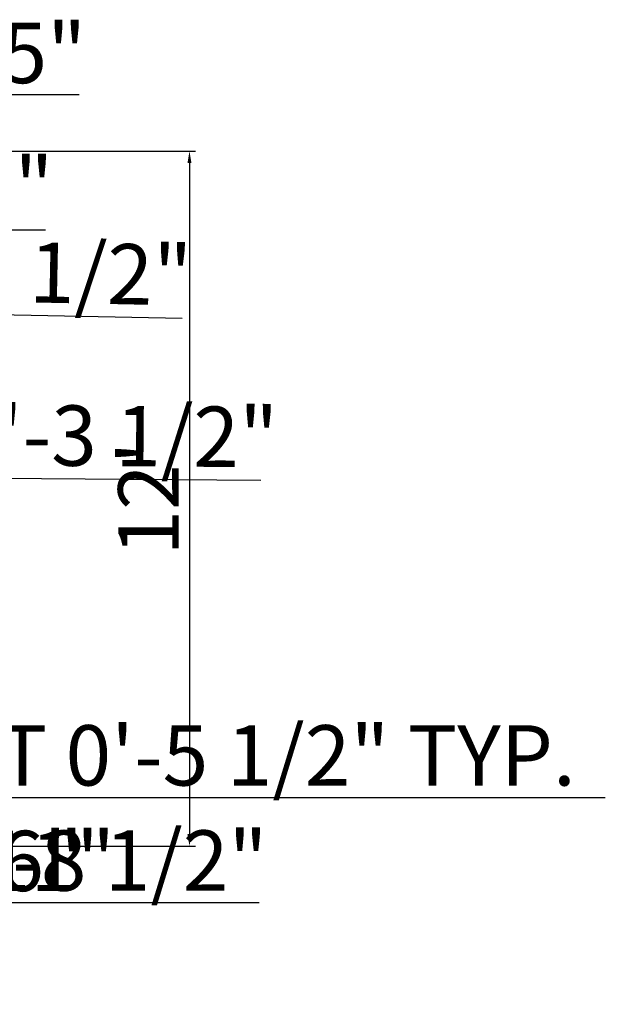
# Model space of a CAD drawing. Units: inches. Extents: x 1545 to 1898, y 1984 to 2198.
# Tile 4 of 4: x 1777 to 1898, y 1984 to 2188. Entities that reach past the tile are written whole.
import ezdxf

# ---------------------------------------------------------------- set-up
doc = ezdxf.new("R2010")
doc.units = ezdxf.units.IN
doc.layers.add('A-ANNO-DIMS', color=2, linetype='Continuous', lineweight=18)
doc.styles.get("Standard").update_dxf_attribs({"font": 'arial.ttf'})
doc.dimstyles.new('ISO-25', dxfattribs={"dimtxt": 12.5, "dimasz": 2.5, "dimexe": 1.25, "dimexo": 0.625, "dimtad": 1, "dimdec": 0, "dimlunit": 3, "dimtxsty": 'Standard', "dimcen": 2.5, "dimadec": 0, "dimazin": 0, "dimtfac": 1, "dimtdec": 0, "dimtmove": 0, "dimatfit": 3, "dimfxl": 1, "dimarcsym": 0})

# ---------------------------------------------------------------- blocks, each defined once
blk = doc.blocks.new('*D5')
at = {"layer": 'A-ANNO-DIMS', "color": 0, "lineweight": -2, "transparency": 16777216}
for p, q in [((1760.62, 2160.51), (1812.93, 2160.51)), ((1811.68, 2158.01), (1811.68, 2019.01)), ((1760.62, 2016.51), (1812.93, 2016.51))]:
    blk.add_line(p, q, dxfattribs=at)
at = {"layer": 'A-ANNO-DIMS', "color": 0, "transparency": 16777216}
for points in [[(1811.27, 2158.01), (1812.1, 2158.01), (1811.68, 2160.51)], [(1811.27, 2019.01), (1812.1, 2019.01), (1811.68, 2016.51)]]:
    blk.add_solid(points, dxfattribs=at)
at = {"layer": 'Defpoints', "color": 0, "transparency": 16777216}
for p in [(1759.99, 2160.51), (1759.99, 2016.51), (1811.68, 2016.51)]:
    blk.add_point(p, dxfattribs=at)
at = {"layer": 'A-ANNO-DIMS', "color": 0, "transparency": 16777216, "insert": (1804.78, 2088.51), "char_height": 12.5, "attachment_point": 5, "rotation": 90}
blk.add_mtext("12'", dxfattribs=at)
blk = doc.blocks.new('*D7')
at = {"layer": 'A-ANNO-DIMS', "color": 0, "lineweight": -2, "transparency": 16777216}
for p, q in [((1657.6, 2026.41), (1657.6, 2027.87)), ((1663.11, 2026.41), (1663.11, 2027.87)), ((1655.1, 2026.62), (1652.6, 2026.62)), ((1657.6, 2026.62), (1663.11, 2026.62)), ((1665.61, 2026.62), (1897.84, 2026.62))]:
    blk.add_line(p, q, dxfattribs=at)
at = {"layer": 'A-ANNO-DIMS', "color": 0, "transparency": 16777216}
for points in [[(1655.1, 2027.03), (1655.1, 2026.2), (1657.6, 2026.62)], [(1665.61, 2027.03), (1665.61, 2026.2), (1663.11, 2026.62)]]:
    blk.add_solid(points, dxfattribs=at)
at = {"layer": 'Defpoints', "color": 0, "transparency": 16777216}
for p in [(1657.6, 2025.79), (1663.11, 2026.62), (1663.11, 2025.79)]:
    blk.add_point(p, dxfattribs=at)
at = {"layer": 'A-ANNO-DIMS', "color": 0, "transparency": 16777216, "insert": (1782.98, 2033.7), "char_height": 12.5, "attachment_point": 5}
blk.add_mtext('SCREEN UNIT 0\'-5 1/2" TYP.', dxfattribs=at)
blk = doc.blocks.new('*D10')
at = {"layer": 'A-ANNO-DIMS', "color": 0, "lineweight": -2, "transparency": 16777216}
for p, q in [((1760.62, 2119.93), (1772.93, 2119.93)), ((1771.68, 2117.43), (1771.68, 2082)), ((1760.62, 2079.5), (1772.93, 2079.5)), ((1771.68, 2079.5), (1771.68, 2013.4))]:
    blk.add_line(p, q, dxfattribs=at)
at = {"layer": 'A-ANNO-DIMS', "color": 0, "transparency": 16777216}
for points in [[(1771.26, 2117.43), (1772.09, 2117.43), (1771.68, 2119.93)], [(1771.26, 2082), (1772.09, 2082), (1771.68, 2079.5)]]:
    blk.add_solid(points, dxfattribs=at)
at = {"layer": 'Defpoints', "color": 0, "transparency": 16777216}
for p in [(1759.99, 2119.93), (1759.99, 2079.5), (1771.68, 2079.5)]:
    blk.add_point(p, dxfattribs=at)
at = {"layer": 'A-ANNO-DIMS', "color": 0, "transparency": 16777216, "insert": (1764.58, 2045.2), "char_height": 12.5, "attachment_point": 5, "rotation": 90}
blk.add_mtext('3\'-4 1/2"', dxfattribs=at)
blk = doc.blocks.new('*D11')
at = {"layer": 'A-ANNO-DIMS', "color": 0, "lineweight": -2, "transparency": 16777216}
for p, q in [((1760.62, 2079.5), (1772.93, 2079.5)), ((1771.68, 2077), (1771.68, 2060.44)), ((1760.62, 2057.94), (1772.93, 2057.94)), ((1771.68, 2057.94), (1771.68, 1993.01))]:
    blk.add_line(p, q, dxfattribs=at)
at = {"layer": 'A-ANNO-DIMS', "color": 0, "transparency": 16777216}
for points in [[(1771.26, 2077), (1772.09, 2077), (1771.68, 2079.5)], [(1771.26, 2060.44), (1772.09, 2060.44), (1771.68, 2057.94)]]:
    blk.add_solid(points, dxfattribs=at)
at = {"layer": 'Defpoints', "color": 0, "transparency": 16777216}
for p in [(1759.99, 2079.5), (1759.99, 2057.94), (1771.68, 2057.94)]:
    blk.add_point(p, dxfattribs=at)
at = {"layer": 'A-ANNO-DIMS', "color": 0, "transparency": 16777216, "insert": (1764.59, 2024.22), "char_height": 12.5, "attachment_point": 5, "rotation": 90}
blk.add_mtext('1\'-9 1/2"', dxfattribs=at)
blk = doc.blocks.new('*D13')
at = {"layer": 'A-ANNO-DIMS', "color": 0, "lineweight": -2, "transparency": 16777216}
for p, q in [((1771.68, 2034.9), (1771.68, 2099.83)), ((1760.62, 2034.9), (1772.93, 2034.9)), ((1771.68, 2019.01), (1771.68, 2032.4)), ((1760.62, 2016.51), (1772.93, 2016.51))]:
    blk.add_line(p, q, dxfattribs=at)
at = {"layer": 'A-ANNO-DIMS', "color": 0, "transparency": 16777216}
for points in [[(1771.26, 2032.4), (1772.09, 2032.4), (1771.68, 2034.9)], [(1771.26, 2019.01), (1772.09, 2019.01), (1771.68, 2016.51)]]:
    blk.add_solid(points, dxfattribs=at)
at = {"layer": 'Defpoints', "color": 0, "transparency": 16777216}
for p in [(1759.99, 2034.9), (1771.68, 2034.9), (1759.99, 2016.51)]:
    blk.add_point(p, dxfattribs=at)
at = {"layer": 'A-ANNO-DIMS', "color": 0, "transparency": 16777216, "insert": (1764.59, 2068.62), "char_height": 12.5, "attachment_point": 5, "rotation": 90}
blk.add_mtext('1\'-6 1/2"', dxfattribs=at)
blk = doc.blocks.new('*D19')
at = {"layer": 'A-ANNO-DIMS', "color": 0, "lineweight": -2, "transparency": 16777216}
for p, q in [((1751.61, 2034.28), (1751.61, 2003.57)), ((1759.99, 2034.28), (1759.99, 2003.57)), ((1754.11, 2004.82), (1757.49, 2004.82)), ((1759.99, 2004.82), (1826.1, 2004.82))]:
    blk.add_line(p, q, dxfattribs=at)
at = {"layer": 'A-ANNO-DIMS', "color": 0, "transparency": 16777216}
for points in [[(1754.11, 2005.24), (1754.11, 2004.41), (1751.61, 2004.82)], [(1757.49, 2005.24), (1757.49, 2004.41), (1759.99, 2004.82)]]:
    blk.add_solid(points, dxfattribs=at)
at = {"layer": 'Defpoints', "color": 0, "transparency": 16777216}
for p in [(1751.61, 2034.9), (1759.99, 2034.9), (1759.99, 2004.82)]:
    blk.add_point(p, dxfattribs=at)
at = {"layer": 'A-ANNO-DIMS', "color": 0, "transparency": 16777216, "insert": (1794.29, 2011.91), "char_height": 12.5, "attachment_point": 5}
blk.add_mtext('0\'-8 1/2"', dxfattribs=at)
blk = doc.blocks.new('*D26')
at = {"layer": 'A-ANNO-DIMS', "color": 0, "lineweight": -2, "transparency": 16777216}
for p, q in [((1722.46, 2150.93), (1722.46, 2173.44)), ((1751.61, 2150.93), (1751.61, 2173.44)), ((1724.96, 2172.19), (1749.11, 2172.19)), ((1751.61, 2172.19), (1788.8, 2172.19))]:
    blk.add_line(p, q, dxfattribs=at)
at = {"layer": 'A-ANNO-DIMS', "color": 0, "transparency": 16777216}
for points in [[(1724.96, 2172.61), (1724.96, 2171.78), (1722.46, 2172.19)], [(1749.11, 2172.61), (1749.11, 2171.78), (1751.61, 2172.19)]]:
    blk.add_solid(points, dxfattribs=at)
at = {"layer": 'Defpoints', "color": 0, "transparency": 16777216}
for p in [(1751.61, 2172.19), (1722.46, 2150.3), (1751.61, 2150.3)]:
    blk.add_point(p, dxfattribs=at)
at = {"layer": 'A-ANNO-DIMS', "color": 0, "transparency": 16777216, "insert": (1771.45, 2179.2), "char_height": 12.5, "attachment_point": 5}
blk.add_mtext('2\'-5"', dxfattribs=at)
blk = doc.blocks.new('*D31')
at = {"layer": 'A-ANNO-DIMS', "color": 0, "lineweight": -2, "transparency": 16777216}
for p, q in [((1752.23, 2150.3), (1772.93, 2150.3)), ((1771.68, 2147.8), (1771.68, 2125.15)), ((1734.02, 2122.65), (1772.93, 2122.65)), ((1771.68, 2122.65), (1771.68, 2056.33))]:
    blk.add_line(p, q, dxfattribs=at)
at = {"layer": 'A-ANNO-DIMS', "color": 0, "transparency": 16777216}
for points in [[(1771.26, 2147.8), (1772.09, 2147.8), (1771.68, 2150.3)], [(1771.26, 2125.15), (1772.09, 2125.15), (1771.68, 2122.65)]]:
    blk.add_solid(points, dxfattribs=at)
at = {"layer": 'Defpoints', "color": 0, "transparency": 16777216}
for p in [(1751.61, 2150.3), (1733.39, 2122.65), (1771.68, 2122.65)]:
    blk.add_point(p, dxfattribs=at)
at = {"layer": 'A-ANNO-DIMS', "color": 0, "transparency": 16777216, "insert": (1764.58, 2088.24), "char_height": 12.5, "attachment_point": 5, "rotation": 90}
blk.add_mtext('2\'-3 1/2"', dxfattribs=at)
blk = doc.blocks.new('*D32')
at = {"layer": 'A-ANNO-DIMS', "color": 0, "lineweight": -2, "transparency": 16777216}
for p, q in [((1734.02, 2122.65), (1772.93, 2122.65)), ((1771.68, 2120.15), (1771.68, 2117.88)), ((1752.23, 2115.38), (1772.93, 2115.38)), ((1771.68, 2115.38), (1771.68, 2049.27))]:
    blk.add_line(p, q, dxfattribs=at)
at = {"layer": 'A-ANNO-DIMS', "color": 0, "transparency": 16777216}
for points in [[(1771.26, 2120.15), (1772.09, 2120.15), (1771.68, 2122.65)], [(1771.26, 2117.88), (1772.09, 2117.88), (1771.68, 2115.38)]]:
    blk.add_solid(points, dxfattribs=at)
at = {"layer": 'Defpoints', "color": 0, "transparency": 16777216}
for p in [(1733.39, 2122.65), (1751.61, 2115.38), (1771.68, 2115.38)]:
    blk.add_point(p, dxfattribs=at)
at = {"layer": 'A-ANNO-DIMS', "color": 0, "transparency": 16777216, "insert": (1764.59, 2081.08), "char_height": 12.5, "attachment_point": 5, "rotation": 90}
blk.add_mtext('0\'-7 1/2"', dxfattribs=at)
blk = doc.blocks.new('*D37')
at = {"layer": 'A-ANNO-DIMS', "color": 0, "lineweight": -2, "transparency": 16777216}
for p, q in [((1733.39, 2065.08), (1733.39, 2003.57)), ((1751.61, 2065.08), (1751.61, 2003.57)), ((1735.89, 2004.82), (1749.11, 2004.82)), ((1751.61, 2004.82), (1787.41, 2004.82))]:
    blk.add_line(p, q, dxfattribs=at)
at = {"layer": 'A-ANNO-DIMS', "color": 0, "transparency": 16777216}
for points in [[(1735.89, 2005.24), (1735.89, 2004.41), (1733.39, 2004.82)], [(1749.11, 2005.24), (1749.11, 2004.41), (1751.61, 2004.82)]]:
    blk.add_solid(points, dxfattribs=at)
at = {"layer": 'Defpoints', "color": 0, "transparency": 16777216}
for p in [(1733.39, 2065.7), (1751.61, 2065.7), (1751.61, 2004.82)]:
    blk.add_point(p, dxfattribs=at)
at = {"layer": 'A-ANNO-DIMS', "color": 0, "transparency": 16777216, "insert": (1770.76, 2011.83), "char_height": 12.5, "attachment_point": 5}
blk.add_mtext('1\'-6"', dxfattribs=at)
blk = doc.blocks.new('*D41')
at = {"layer": 'A-ANNO-DIMS', "color": 0, "lineweight": -2, "transparency": 16777216}
for p, q in [((1737.08, 2085.23), (1737.08, 2003.57)), ((1748.11, 2085.23), (1748.11, 2003.57)), ((1739.58, 2004.82), (1745.61, 2004.82)), ((1748.11, 2004.82), (1794.8, 2004.82))]:
    blk.add_line(p, q, dxfattribs=at)
at = {"layer": 'A-ANNO-DIMS', "color": 0, "transparency": 16777216}
for points in [[(1739.58, 2005.24), (1739.58, 2004.41), (1737.08, 2004.82)], [(1745.61, 2005.24), (1745.61, 2004.41), (1748.11, 2004.82)]]:
    blk.add_solid(points, dxfattribs=at)
at = {"layer": 'Defpoints', "color": 0, "transparency": 16777216}
for p in [(1737.08, 2085.86), (1748.11, 2085.86), (1748.11, 2004.82)]:
    blk.add_point(p, dxfattribs=at)
at = {"layer": 'A-ANNO-DIMS', "color": 0, "transparency": 16777216, "insert": (1772.71, 2011.83), "char_height": 12.5, "attachment_point": 5}
blk.add_mtext('0\'-11"', dxfattribs=at)
blk = doc.blocks.new('*D45')
at = {"layer": 'A-ANNO-DIMS', "color": 0, "lineweight": -2, "transparency": 16777216}
for p, q in [((1693.9, 2144.11), (1691.4, 2144.11)), ((1696.4, 2144.11), (1702.37, 2144.11)), ((1781.85, 2144.11), (1704.87, 2144.11))]:
    blk.add_line(p, q, dxfattribs=at)
at = {"layer": 'A-ANNO-DIMS', "color": 0, "transparency": 16777216}
for points in [[(1693.9, 2144.53), (1693.9, 2143.7), (1696.4, 2144.11)], [(1704.87, 2144.53), (1704.87, 2143.7), (1702.37, 2144.11)]]:
    blk.add_solid(points, dxfattribs=at)
at = {"layer": 'Defpoints', "color": 0, "transparency": 16777216}
for p in [(1696.4, 2144.11), (1702.37, 2144.11)]:
    blk.add_point(p, dxfattribs=at)
at = {"layer": 'A-ANNO-DIMS', "color": 0, "transparency": 16777216, "insert": (1744.61, 2151.47), "char_height": 12.5, "attachment_point": 5, "rotation": 359.999}
blk.add_mtext('2X ∅0\'-6"', dxfattribs=at)
blk = doc.blocks.new('*D47')
at = {"layer": 'A-ANNO-DIMS', "color": 0, "lineweight": -2, "transparency": 16777216}
for p, q in [((1695.76, 2128.1), (1693.26, 2128.15)), ((1698.26, 2128.05), (1701.6, 2127.98)), ((1810.19, 2125.79), (1704.1, 2127.93))]:
    blk.add_line(p, q, dxfattribs=at)
at = {"layer": 'A-ANNO-DIMS', "color": 0, "transparency": 16777216}
for points in [[(1695.76, 2128.51), (1695.75, 2127.68), (1698.26, 2128.05)], [(1704.11, 2128.35), (1704.09, 2127.51), (1701.6, 2127.98)]]:
    blk.add_solid(points, dxfattribs=at)
at = {"layer": 'Defpoints', "color": 0, "transparency": 16777216}
for p in [(1698.26, 2128.05), (1701.6, 2127.98)]:
    blk.add_point(p, dxfattribs=at)
at = {"layer": 'A-ANNO-DIMS', "color": 0, "transparency": 16777216, "insert": (1758.54, 2134.19), "char_height": 12.5, "attachment_point": 5, "rotation": 358.8454}
blk.add_mtext('2X ∅0\'-3 1/2"', dxfattribs=at)
blk = doc.blocks.new('*D48')
at = {"layer": 'A-ANNO-DIMS', "color": 0, "lineweight": -2, "transparency": 16777216}
for p, q in [((1738.41, 2092.96), (1735.91, 2092.98)), ((1740.91, 2092.94), (1744.28, 2092.91)), ((1826.49, 2092.27), (1746.78, 2092.89))]:
    blk.add_line(p, q, dxfattribs=at)
at = {"layer": 'A-ANNO-DIMS', "color": 0, "transparency": 16777216}
for points in [[(1738.42, 2093.37), (1738.41, 2092.54), (1740.91, 2092.94)], [(1746.79, 2093.31), (1746.78, 2092.47), (1744.28, 2092.91)]]:
    blk.add_solid(points, dxfattribs=at)
at = {"layer": 'Defpoints', "color": 0, "transparency": 16777216}
for p in [(1740.91, 2092.94), (1744.28, 2092.91)]:
    blk.add_point(p, dxfattribs=at)
at = {"layer": 'A-ANNO-DIMS', "color": 0, "transparency": 16777216, "insert": (1787.94, 2099.93), "char_height": 12.5, "attachment_point": 5, "rotation": 359.5524}
blk.add_mtext('∅0\'-3 1/2"', dxfattribs=at)

msp = doc.modelspace()

# ---------------------------------------------------------------- dimensions: what is measured, and where the dimension line sits
at = {"layer": 'A-ANNO-DIMS'}
for base, p1, p2, picture, middle in [((1751.6089, 2172.1934), (1722.4582, 2150.3018), (1751.6089, 2150.3018), '*D26', (1771.4546, 2179.2005)), ((1748.11, 2004.82), (1737.08, 2085.86), (1748.11, 2085.86), '*D41', (1772.71, 2011.83)), ((1751.61, 2004.82), (1733.39, 2065.7), (1751.61, 2065.7), '*D37', (1770.76, 2011.83)), ((1759.99, 2004.82), (1751.61, 2034.9), (1759.99, 2034.9), '*D19', (1794.29, 2011.91))]:
    dim = msp.add_linear_dim(base=base, p1=p1, p2=p2, dimstyle='ISO-25', override={"dimdec": 1, "dimlfac": 1, "dimrnd": 0, "dimzin": 1, "dimdsep": 46, "dimlunit": 4, "dimfrac": 2}, dxfattribs=at)
    dim.commit()
    dim.dimension.update_dxf_attribs({"geometry": picture, "text_midpoint": middle})
for p1, p2, picture, middle in [((1696.4, 2144.11), (1702.37, 2144.11), '*D45', (1744.61, 2144.11)), ((1698.26, 2128.05), (1701.6, 2127.98), '*D47', (1758.39, 2126.84))]:
    dim = msp.add_diameter_dim_2p(p1=p1, p2=p2, text='2X <>', dimstyle='ISO-25', override={"dimdec": 1, "dimlfac": 1, "dimrnd": 0, "dimzin": 1, "dimdsep": 46, "dimlunit": 4, "dimfrac": 2}, dxfattribs=at)
    dim.commit()
    dim.dimension.update_dxf_attribs({"geometry": picture, "text_midpoint": middle})
for base, p1, p2, override, picture, middle in [((1811.68, 2016.51), (1759.99, 2160.51), (1759.99, 2016.51), {"dimclrd": 0, "dimclre": 0, "dimclrt": 0}, '*D5', (1804.78, 2088.51)), ((1771.6756, 2122.652), (1751.6089, 2150.3018), (1733.3924, 2122.652), {"dimdec": 1, "dimlfac": 1, "dimrnd": 0, "dimzin": 1, "dimdsep": 46, "dimlunit": 4, "dimfrac": 2}, '*D31', (1764.5832, 2088.2429)), ((1771.68, 2115.38), (1733.39, 2122.65), (1751.61, 2115.38), {"dimdec": 1, "dimlfac": 1, "dimrnd": 0, "dimzin": 1, "dimdsep": 46, "dimlunit": 4, "dimfrac": 2}, '*D32', (1764.59, 2081.08)), ((1771.68, 2079.5), (1759.99, 2119.93), (1759.99, 2079.5), {"dimdec": 1, "dimlfac": 1, "dimrnd": 0, "dimzin": 1, "dimdsep": 46, "dimlunit": 4, "dimfrac": 2}, '*D10', (1764.58, 2045.2)), ((1771.68, 2034.9), (1759.99, 2016.51), (1759.99, 2034.9), {"dimdec": 1, "dimlfac": 1, "dimrnd": 0, "dimzin": 1, "dimdsep": 46, "dimlunit": 4, "dimfrac": 2}, '*D13', (1764.59, 2068.62)), ((1771.68, 2057.94), (1759.99, 2079.5), (1759.99, 2057.94), {"dimdec": 1, "dimlfac": 1, "dimrnd": 0, "dimzin": 1, "dimdsep": 46, "dimlunit": 4, "dimfrac": 2}, '*D11', (1764.59, 2024.22))]:
    dim = msp.add_linear_dim(base=base, p1=p1, p2=p2, angle=90, dimstyle='ISO-25', override=override, dxfattribs=at)
    dim.commit()
    dim.dimension.update_dxf_attribs({"geometry": picture, "text_midpoint": middle})
dim = msp.add_diameter_dim_2p(p1=(1740.91, 2092.94), p2=(1744.28, 2092.91), dimstyle='ISO-25', override={"dimdec": 1, "dimlfac": 1, "dimrnd": 0, "dimzin": 1, "dimdsep": 46, "dimlunit": 4, "dimfrac": 2}, dxfattribs=at)
dim.commit()
dim.dimension.update_dxf_attribs({"geometry": '*D48', "text_midpoint": (1787.89, 2092.57)})
dim = msp.add_linear_dim(base=(1663.11, 2026.62), p1=(1657.6, 2025.79), p2=(1663.11, 2025.79), text='SCREEN UNIT <> TYP.', dimstyle='ISO-25', override={"dimdec": 1, "dimlfac": 1, "dimrnd": 0, "dimzin": 1, "dimdsep": 46, "dimlunit": 4, "dimfrac": 2}, dxfattribs=at)
dim.commit()
dim.dimension.update_dxf_attribs({"geometry": '*D7', "text_midpoint": (1782.98, 2033.7)})

doc.saveas('drawing.dxf')
